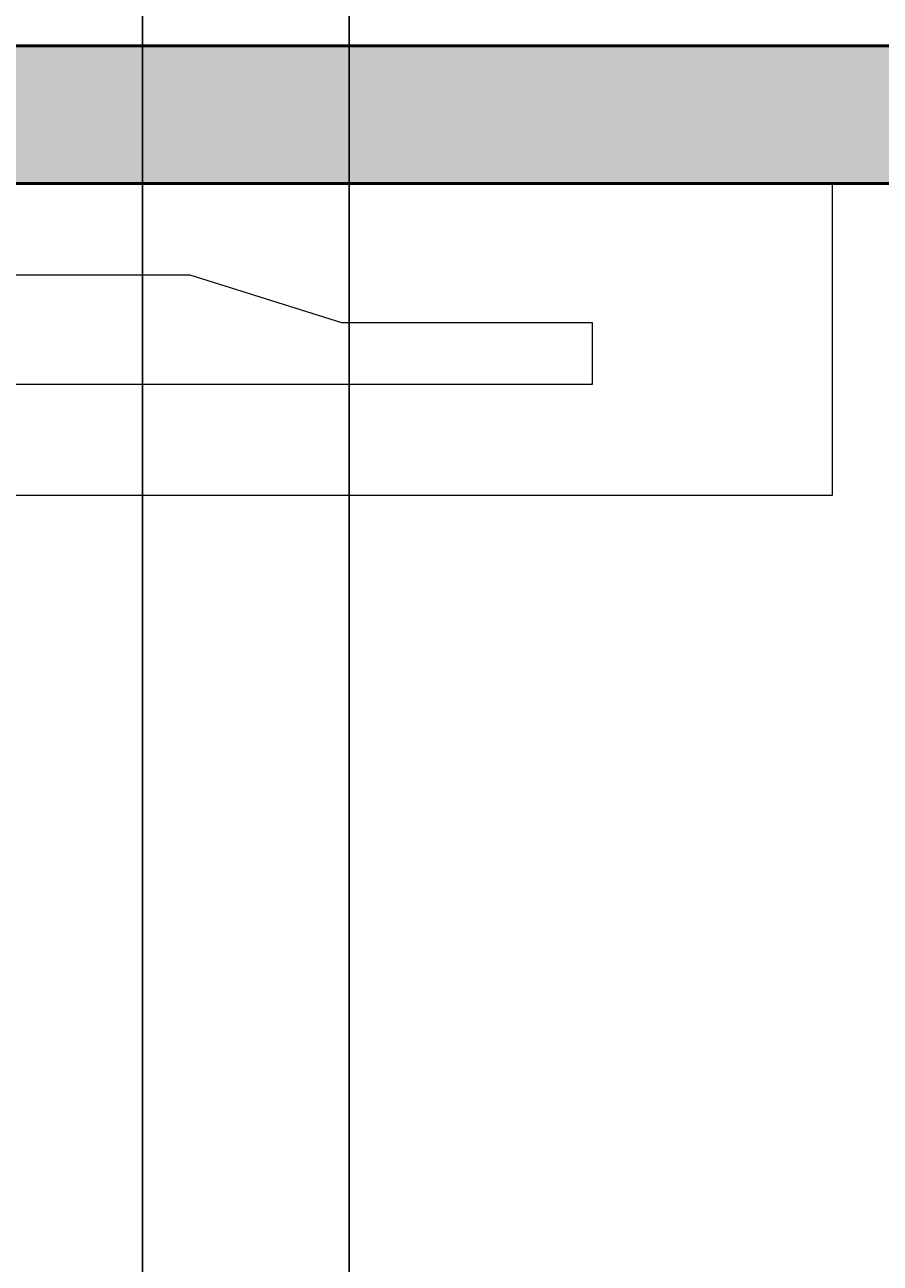
# Model space of a CAD drawing. Units: inches. Extents: x 2231 to 2461, y 2045 to 2455.
# Tile 52 of 95: x 2295 to 2320, y 2271 to 2307. Entities that reach past the tile are written whole.
import ezdxf

# ---------------------------------------------------------------- set-up
doc = ezdxf.new("R2010")
doc.units = ezdxf.units.IN
for name, color, linetype, lineweight in [('A-ANNO-DIMS', 2, 'Continuous', 18), ('A-EQPM', 8, 'Continuous', 18), ('A-FURN', 9, 'Continuous', 18), ('A-WALL', 7, 'Continuous', 50)]:
    doc.layers.add(name, color=color, linetype=linetype, lineweight=lineweight)
doc.layers.add('A-WALL-PATT', color=18, linetype='Continuous', lineweight=13, true_color=0x000000)
doc.styles.get("Standard").update_dxf_attribs({"font": 'arial.ttf'})
doc.dimstyles.get("Standard").update_dxf_attribs({"dimtxt": 0.18, "dimasz": 0.18, "dimexe": 0.18, "dimexo": 0.0625, "dimgap": 0.09, "dimtad": 0, "dimtih": 1, "dimtoh": 1, "dimdec": 4, "dimzin": 0, "dimdsep": 46, "dimtxsty": 'Standard', "dimcen": 0.09, "dimadec": 0, "dimazin": 0, "dimtfac": 1, "dimtdec": 4, "dimtofl": 0, "dimtmove": 0, "dimatfit": 3, "dimfxl": 1, "dimtolj": 1, "dimtzin": 0, "dimarcsym": 0})

# ---------------------------------------------------------------- blocks, each defined once
blk = doc.blocks.new('*D49')
at = {"layer": 'A-ANNO-DIMS', "color": 0, "lineweight": -2, "transparency": 16777216}
for p, q in [((2298.794, 2182.895), (2298.794, 2454.645)), ((2298.974, 2454.465), (2301.644, 2454.465)), ((2304.614, 2454.465), (2301.943, 2454.465)), ((2304.794, 2182.895), (2304.794, 2454.645))]:
    blk.add_line(p, q, dxfattribs=at)
at = {"layer": 'A-ANNO-DIMS', "color": 0, "transparency": 16777216}
for points in [[(2298.974, 2454.495), (2298.974, 2454.435), (2298.794, 2454.465)], [(2304.614, 2454.495), (2304.614, 2454.435), (2304.794, 2454.465)]]:
    blk.add_solid(points, dxfattribs=at)
at = {"layer": 'Defpoints', "color": 0, "transparency": 16777216}
for p in [(2304.794, 2454.465), (2298.794, 2182.833), (2304.794, 2182.833)]:
    blk.add_point(p, dxfattribs=at)
at = {"layer": 'A-ANNO-DIMS', "color": 0, "transparency": 16777216, "insert": (2301.794, 2454.465), "char_height": 0.18, "attachment_point": 5}
blk.add_mtext('\\A1;6', dxfattribs=at)
blk = doc.blocks.new('*D50')
at = {"layer": 'A-ANNO-DIMS', "color": 0, "lineweight": -2, "transparency": 16777216}
for p, q in [((2304.794, 2182.895), (2304.794, 2454.645)), ((2304.974, 2454.465), (2319.575, 2454.465)), ((2334.614, 2454.465), (2320.012, 2454.465)), ((2334.794, 2182.895), (2334.794, 2454.645))]:
    blk.add_line(p, q, dxfattribs=at)
at = {"layer": 'A-ANNO-DIMS', "color": 0, "transparency": 16777216}
for points in [[(2304.974, 2454.495), (2304.974, 2454.435), (2304.794, 2454.465)], [(2334.614, 2454.495), (2334.614, 2454.435), (2334.794, 2454.465)]]:
    blk.add_solid(points, dxfattribs=at)
at = {"layer": 'Defpoints', "color": 0, "transparency": 16777216}
for p in [(2334.794, 2454.465), (2304.794, 2182.833), (2334.794, 2182.833)]:
    blk.add_point(p, dxfattribs=at)
at = {"layer": 'A-ANNO-DIMS', "color": 0, "transparency": 16777216, "insert": (2319.794, 2454.465), "char_height": 0.18, "attachment_point": 5}
blk.add_mtext('\\A1;30', dxfattribs=at)
blk = doc.blocks.new('*D51')
at = {"layer": 'A-ANNO-DIMS', "color": 0, "lineweight": -2, "transparency": 16777216}
for p, q in [((2258.794, 2306.77), (2258.794, 2044.803)), ((2330.794, 2306.77), (2330.794, 2044.803)), ((2258.974, 2044.983), (2294.576, 2044.983)), ((2330.614, 2044.983), (2295.011, 2044.983))]:
    blk.add_line(p, q, dxfattribs=at)
at = {"layer": 'A-ANNO-DIMS', "color": 0, "transparency": 16777216}
for points in [[(2258.974, 2045.013), (2258.974, 2044.953), (2258.794, 2044.983)], [(2330.614, 2045.013), (2330.614, 2044.953), (2330.794, 2044.983)]]:
    blk.add_solid(points, dxfattribs=at)
at = {"layer": 'Defpoints', "color": 0, "transparency": 16777216}
for p in [(2258.794, 2306.833), (2330.794, 2306.833), (2330.794, 2044.983)]:
    blk.add_point(p, dxfattribs=at)
at = {"layer": 'A-ANNO-DIMS', "color": 0, "transparency": 16777216, "insert": (2294.794, 2044.983), "char_height": 0.18, "attachment_point": 5}
blk.add_mtext('\\A1;72', dxfattribs=at)

msp = doc.modelspace()

# ---------------------------------------------------------------- hatches: boundary and pattern name
at = {"layer": 'A-WALL-PATT'}
h = msp.add_hatch(color=256, dxfattribs=at)
h.dxf.hatch_style = 1
h.paths.add_polyline_path([(2441.7935, 2269.1535), (2432.7935, 2269.1535), (2432.7935, 2186.8328), (2396.7935, 2186.8328), (2396.7935, 2286.8328), (2394.7935, 2286.8328), (2394.7935, 2186.8328), (2334.7935, 2186.8328), (2334.7935, 2182.8328), (2432.7935, 2182.8328), (2432.7935, 2072.8328), (2416.6639, 2072.8328), (2416.6639, 2063.8328), (2441.7935, 2063.8328)])
h.paths.add_polyline_path([(2368.6639, 2072.8328), (2367.04, 2072.8328), (2330.7942, 2072.8328), (2330.7397, 2063.8328), (2368.6639, 2063.8328)])
h.paths.add_polyline_path([(2300.7392, 2068.3328), (2300.7392, 2072.8328), (2298.7935, 2072.8328), (2294.7935, 2072.8328), (2258.7935, 2072.8328), (2258.7935, 2120.8328), (2294.7935, 2120.8328), (2298.7935, 2120.8328), (2298.7935, 2128.8328), (2294.7935, 2128.8328), (2294.7935, 2124.8328), (2258.7935, 2124.8328), (2258.7935, 2182.8328), (2294.7935, 2182.8328), (2294.7935, 2174.8328), (2298.7935, 2174.8328), (2298.7935, 2182.8328), (2304.7935, 2182.8328), (2304.7935, 2186.8328), (2258.7935, 2186.8328), (2258.7935, 2221.999), (2249.7935, 2221.999), (2249.7935, 2063.8328), (2300.7392, 2063.8328)])
h.paths.add_polyline_path([(2391.9338, 2435.8328), (2333.82, 2435.8328), (2333.82, 2426.8328), (2368.7935, 2426.8328), (2368.7935, 2374.9508), (2368.7935, 2370.8328), (2372.3935, 2370.8328), (2372.7935, 2370.8328), (2372.7935, 2426.8328), (2391.9338, 2426.8328)])
h.paths.add_polyline_path([(2441.7935, 2435.8328), (2415.9338, 2435.8328), (2415.9338, 2426.8328), (2432.7935, 2426.8328), (2432.7935, 2334.8328), (2372.7935, 2334.8328), (2372.7935, 2346.8328), (2368.7935, 2346.8328), (2368.7935, 2306.8328), (2360.7935, 2306.8328), (2360.7935, 2302.8328), (2368.7935, 2302.8328), (2372.7935, 2302.8328), (2372.7935, 2330.8328), (2432.7935, 2330.8328), (2432.7935, 2317.1535), (2441.7935, 2317.1535)])
h.paths.add_polyline_path([(2285.82, 2435.8328), (2249.7935, 2435.8328), (2249.7935, 2269.999), (2258.7935, 2269.999), (2258.7935, 2302.8328), (2318.8168, 2302.8328), (2330.7935, 2302.8328), (2330.7935, 2306.8328), (2258.7935, 2306.8328), (2258.7935, 2426.8328), (2285.82, 2426.8328)])

# ---------------------------------------------------------------- linework, layer by layer
at = {"layer": 'A-EQPM'}
msp.add_line((2300.1765, 2300.1814), (2304.5787, 2298.7991), dxfattribs=at)
for points in [[(2275.7007, 2300.1814), (2300.1765, 2300.1814)], [(2304.5787, 2298.7991), (2311.8486, 2298.7991), (2311.8486, 2296.9979), (2264.0286, 2296.9979), (2264.0286, 2298.7991), (2271.2638, 2298.7991)]]:
    msp.add_lwpolyline(points, dxfattribs=at)
at = {"layer": 'A-FURN'}
msp.add_lwpolyline([(2258.7935, 2302.8328), (2318.8168, 2302.8328), (2318.8168, 2293.7759), (2258.7935, 2293.7759)], close=True, dxfattribs=at)
at = {"layer": 'A-WALL'}
for p, q in [((2258.7935, 2306.8328), (2330.7935, 2306.8328)), ((2258.7935, 2302.8328), (2330.7935, 2302.8328))]:
    msp.add_line(p, q, dxfattribs=at)

# ---------------------------------------------------------------- dimensions: what is measured, and where the dimension line sits
at = {"layer": 'A-ANNO-DIMS'}
for base, p1, p2, picture, middle in [((2304.7935, 2454.4653), (2298.7935, 2182.8328), (2304.7935, 2182.8328), '*D49', (2301.7935, 2454.4653)), ((2334.7935, 2454.4653), (2304.7935, 2182.8328), (2334.7935, 2182.8328), '*D50', (2319.7935, 2454.4653)), ((2330.7935, 2044.9825), (2258.7935, 2306.8328), (2330.7935, 2306.8328), '*D51', (2294.7935, 2044.9825))]:
    dim = msp.add_linear_dim(base=base, p1=p1, p2=p2, dimstyle='Standard', override={"dimdec": 0, "dimlfac": 1, "dimrnd": 0, "dimzin": 0, "dimdsep": 46, "dimlunit": 2}, dxfattribs=at)
    dim.commit()
    dim.dimension.update_dxf_attribs({"geometry": picture, "text_midpoint": middle})

doc.saveas('drawing.dxf')
